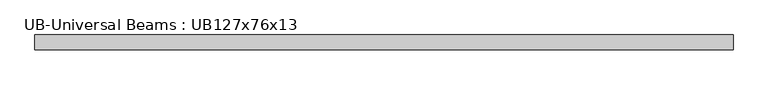
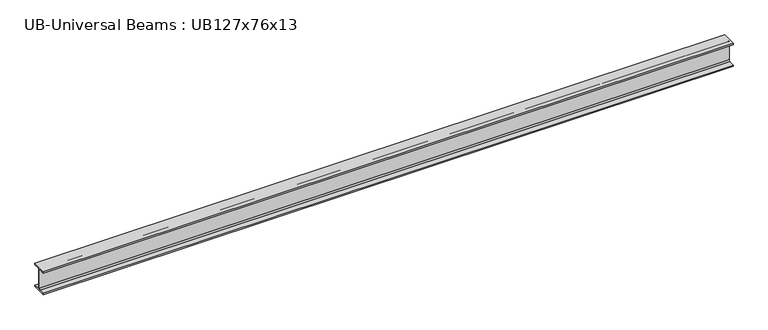
"""IFC4 building model written with IfcOpenShell, lengths in millimetres: member geometry, UB-Universal Beams : UB127x76x13."""

from ifc_helpers import new_model, si_unit, point, frame, frame_2d, origin, place, context, project, spatial, polyline, circle_curve, trimmed, segment, composite_curve, outline, extrude, source, transform, mapped, element, save


def ub_universal_beams_ub127x76x13_6b492b77(model_context):
    return source(origin(), model_context, "Body", "SweptSolid", [
        extrude(outline(composite_curve([segment(polyline([(-38.0, -55.9), (-9.6, -55.9)]), True, "CONTINUOUS"), segment(trimmed(circle_curve(frame_2d((-9.6, -48.3)), 7.6), [point((-9.6, -55.9))], [point((-2.0, -48.3))], True, "CARTESIAN"), True, "CONTINUOUS"), segment(polyline([(-2.0, -48.3), (-2.0, 48.3)]), True, "CONTINUOUS"), segment(trimmed(circle_curve(frame_2d((-9.6, 48.3)), 7.6), [point((-2.0, 48.3))], [point((-9.6, 55.9))], True, "CARTESIAN"), True, "CONTINUOUS"), segment(polyline([(-9.6, 55.9), (-38.0, 55.9), (-38.0, 63.5), (38.0, 63.5), (38.0, 55.9), (9.6, 55.9)]), True, "CONTINUOUS"), segment(trimmed(circle_curve(frame_2d((9.6, 48.3)), 7.6), [point((9.6, 55.9))], [point((2.0, 48.3))], True, "CARTESIAN"), True, "CONTINUOUS"), segment(polyline([(2.0, 48.3), (2.0, -48.3)]), True, "CONTINUOUS"), segment(trimmed(circle_curve(frame_2d((9.6, -48.3)), 7.6), [point((2.0, -48.3))], [point((9.6, -55.9))], True, "CARTESIAN"), True, "CONTINUOUS"), segment(polyline([(9.6, -55.9), (38.0, -55.9), (38.0, -63.5), (-38.0, -63.5), (-38.0, -55.9)]), True, "CONTINUOUS")], self_intersect=False)), frame((-2004.55, 0.0, 0.0), z_axis=(1.0, 0.0, 0.0), x_axis=(0.0, 1.0, 0.0)), (0.0, 0.0, 1.0), 3585.6),
    ])


if __name__ == "__main__":
    model = new_model("IFC4")
    model_context = context("Model", 3, world=origin())
    ifc_project = project(units=[si_unit("LENGTHUNIT", "METRE", prefix="MILLI")], contexts=[model_context])
    site = spatial("IfcSite", under=ifc_project)
    building = spatial("IfcBuilding", under=site)
    placement = place(None, origin())
    ub_universal_beams_ub127x76x13_shape = ub_universal_beams_ub127x76x13_6b492b77(model_context)
    element("IfcMember", 1, ObjectType="UB-Universal Beams : UB127x76x13", at=placement, inside=building, context=model_context, shape_type="MappedRepresentation", body=[
        mapped(ub_universal_beams_ub127x76x13_shape, transform((0.0, 0.0, 0.0), x_axis=(1.0, 0.0, 0.0), y_axis=(0.0, 1.0, 0.0), z_axis=(0.0, 0.0, 1.0))),
    ])
    save(model, "model.ifc")

# Revit data of these elements
# Type "UB-Universal Beams : UB127x76x13"
#   Section Name Key = "UB127X76X13"
#   Width = 7.6 cm
#   Web Thickness = 0.4 cm
#   Web Fillet = 0.76 cm
#   Warping Constant = 2000.0 cm⁶
#   Torsional Moment of Inertia = 2.85 cm⁴
#   Section Area = 16.5 cm²
#   Plastic Modulus weak axis = 22.6 cm³
#   Plastic Modulus strong axis = 84.2 cm³
#   Nominal Weight = 13.00 kgf/m
#   Moment of Inertia weak axis = 55.70 cm⁴
#   Moment of Inertia strong axis = 473.00 cm⁴
#   Height = 12.7 cm
#   Flange Thickness = 0.76 cm
#   Elastic Modulus weak axis = 14.7 cm³
#   Elastic Modulus strong axis = 74.6 cm³
#   Centroid Vertical = 6.35 cm
#   Centroid Horizontal = 3.8 cm
#   Bolt Spacing = 4.0 cm
#   Length [instance default] = 1.5 m
#   Structural Material [instance default] = Metal - Steel 43-275
#   Type Comments = ""
#   Assembly Code = ""
# Element 1 (IfcMember, "UB-Universal Beams : UB127x76x13")
#   Materials on its faces: "Metal - Steel 43-275"
# Materials
#   "Metal - Steel 43-275": class "Metal", colour RGB 247 247 247, transparency 0, Cost = 0
